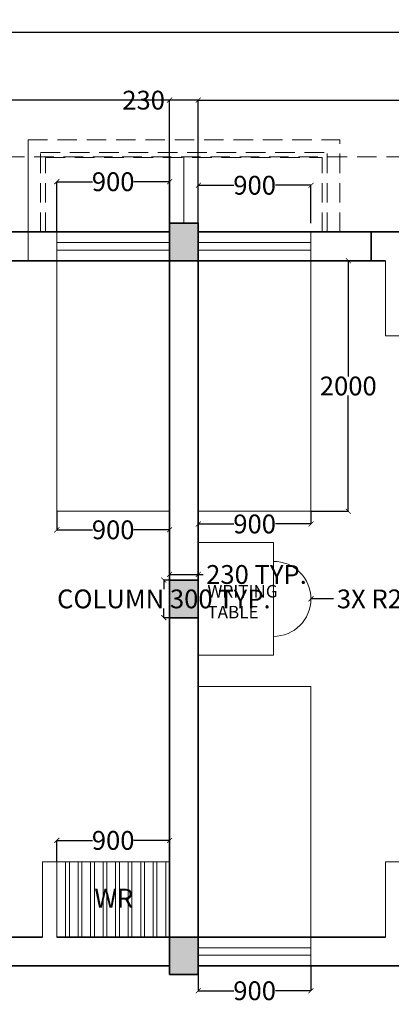
# Model space of a CAD drawing. Units: millimetres. Extents: x 32888 to 53184, y 27889 to 39696.
# Tile 3 of 6: x 38202 to 41170, y 31834 to 39696. Entities that reach past the tile are written whole.
import ezdxf

# ---------------------------------------------------------------- set-up
doc = ezdxf.new("R2010")
doc.units = ezdxf.units.MM
doc.header["$LTSCALE"] = 50
doc.header["$MEASUREMENT"] = 0
doc.linetypes.add('HIDDEN2', pattern=[0.1875, 0.125, -0.0625])
for name, color, linetype, lineweight in [('A-ANNO-DIMS', 2, 'Continuous', 18), ('A-ANNO-TEXT', 7, 'Continuous', 18), ('A-COLS', 1, 'Continuous', 35), ('A-COLS-PATT', 18, 'Continuous', 18), ('A-FURN', 8, 'Continuous', 18), ('A-FURN-CASE', 8, 'Continuous', 18), ('A-GLAZ', 4, 'Continuous', 18), ('A-ROOF', 8, 'Continuous', 18), ('A-ROOF-OVHD', 8, 'HIDDEN2', 18), ('A-WALL', 7, 'Continuous', 35)]:
    doc.layers.add(name, color=color, linetype=linetype, lineweight=lineweight)
doc.styles.get("Standard").update_dxf_attribs({"font": 'arial.ttf'})
doc.dimstyles.get("Standard").update_dxf_attribs({"dimtxt": 150, "dimasz": 40, "dimexe": 0.18, "dimexo": 0.0625, "dimgap": 0.09, "dimtad": 0, "dimtih": 1, "dimtoh": 1, "dimdec": 0, "dimzin": 0, "dimdsep": 46, "dimtxsty": 'Standard', "dimblk": 'ARCHTICK', "dimcen": 0, "dimadec": 0, "dimazin": 0, "dimtfac": 1, "dimtdec": 0, "dimtofl": 0, "dimtmove": 0, "dimatfit": 3, "dimldrblk": 'ARCHTICK', "dimfxl": 1, "dimtolj": 1, "dimtzin": 0, "dimarcsym": 1})

# ---------------------------------------------------------------- blocks, each defined once
blk = doc.blocks.new('_ArchTick')
at = {"color": 0, "linetype": 'ByBlock', "const_width": 0.15}
blk.add_lwpolyline([(-0.5, -0.5), (0.5, 0.5)], dxfattribs=at)
blk = doc.blocks.new('*D14')
at = {"layer": 'A-ANNO-DIMS', "color": 0, "lineweight": -2, "ltscale": 50, "transparency": 16777216}
for p, q in [((38498.9, 32971.1), (38498.9, 33143.1)), ((38498.9, 33142.9), (38783.4, 33142.9)), ((39398.9, 33142.9), (39114.5, 33142.9)), ((39398.9, 32971.1), (39398.9, 33143.1))]:
    blk.add_line(p, q, dxfattribs=at)
at = {"layer": 'Defpoints', "color": 0, "ltscale": 50, "transparency": 16777216}
for p in [(39398.9, 33142.9), (38498.9, 32971), (39398.9, 32971)]:
    blk.add_point(p, dxfattribs=at)
at = {"layer": 'A-ANNO-DIMS', "color": 0, "lineweight": -2, "ltscale": 50, "transparency": 16777216, "xscale": 40, "yscale": 40, "zscale": 40, "rotation": 180}
blk.add_blockref('_ArchTick', (38498.9, 33142.9), dxfattribs=at)
at = {"layer": 'A-ANNO-DIMS', "color": 0, "lineweight": -2, "ltscale": 50, "transparency": 16777216, "xscale": 40, "yscale": 40, "zscale": 40}
blk.add_blockref('_ArchTick', (39398.9, 33142.9), dxfattribs=at)
at = {"layer": 'A-ANNO-DIMS', "color": 0, "ltscale": 50, "transparency": 16777216, "insert": (38948.9, 33142.9), "char_height": 150, "attachment_point": 5}
blk.add_mtext('\\A1;900', dxfattribs=at)
blk = doc.blocks.new('*D18')
at = {"layer": 'A-ANNO-DIMS', "color": 0, "lineweight": -2, "ltscale": 50, "transparency": 16777216}
for p, q in [((39628.9, 32140.9), (39628.9, 31942.1)), ((40528.9, 32140.9), (40528.9, 31942.1)), ((39628.9, 31942.3), (39913.4, 31942.3)), ((40528.9, 31942.3), (40244.5, 31942.3))]:
    blk.add_line(p, q, dxfattribs=at)
at = {"layer": 'Defpoints', "color": 0, "ltscale": 50, "transparency": 16777216}
for p in [(39628.9, 32141), (40528.9, 32141), (40528.9, 31942.3)]:
    blk.add_point(p, dxfattribs=at)
at = {"layer": 'A-ANNO-DIMS', "color": 0, "lineweight": -2, "ltscale": 50, "transparency": 16777216, "xscale": 40, "yscale": 40, "zscale": 40, "rotation": 180}
blk.add_blockref('_ArchTick', (39628.9, 31942.3), dxfattribs=at)
at = {"layer": 'A-ANNO-DIMS', "color": 0, "lineweight": -2, "ltscale": 50, "transparency": 16777216, "xscale": 40, "yscale": 40, "zscale": 40}
blk.add_blockref('_ArchTick', (40528.9, 31942.3), dxfattribs=at)
at = {"layer": 'A-ANNO-DIMS', "color": 0, "ltscale": 50, "transparency": 16777216, "insert": (40078.9, 31942.3), "char_height": 150, "attachment_point": 5}
blk.add_mtext('\\A1;900', dxfattribs=at)
blk = doc.blocks.new('*D36')
at = {"layer": 'A-ANNO-DIMS', "color": 0, "lineweight": -2, "ltscale": 50, "transparency": 16777216}
for p, q in [((40529, 37771), (40826.9, 37771)), ((40826.7, 37771), (40826.7, 36847.7)), ((40826.7, 35771), (40826.7, 36694.3)), ((40529, 35771), (40826.9, 35771))]:
    blk.add_line(p, q, dxfattribs=at)
at = {"layer": 'Defpoints', "color": 0, "ltscale": 50, "transparency": 16777216}
for p in [(40528.9, 37771), (40826.7, 37771), (40528.9, 35771)]:
    blk.add_point(p, dxfattribs=at)
at = {"layer": 'A-ANNO-DIMS', "color": 0, "lineweight": -2, "ltscale": 50, "transparency": 16777216, "xscale": 40, "yscale": 40, "zscale": 40}
for p, rotation in [((40826.7, 37771), 90), ((40826.7, 35771), 270)]:
    blk.add_blockref('_ArchTick', p, dxfattribs=dict(at, rotation=rotation))
at = {"layer": 'A-ANNO-DIMS', "color": 0, "ltscale": 50, "transparency": 16777216, "insert": (40826.7, 36771), "char_height": 150, "attachment_point": 5}
blk.add_mtext('\\A1;2000', dxfattribs=at)
blk = doc.blocks.new('*D37')
at = {"layer": 'A-ANNO-DIMS', "color": 0, "lineweight": -2, "ltscale": 50, "transparency": 16777216}
for p, q in [((39628.9, 35770.9), (39628.9, 35669.2)), ((40528.9, 35770.9), (40528.9, 35669.2)), ((39628.9, 35669.3), (39913.4, 35669.3)), ((40528.9, 35669.3), (40244.5, 35669.3))]:
    blk.add_line(p, q, dxfattribs=at)
at = {"layer": 'Defpoints', "color": 0, "ltscale": 50, "transparency": 16777216}
for p in [(39628.9, 35771), (40528.9, 35771), (39628.9, 35669.3)]:
    blk.add_point(p, dxfattribs=at)
at = {"layer": 'A-ANNO-DIMS', "color": 0, "lineweight": -2, "ltscale": 50, "transparency": 16777216, "xscale": 40, "yscale": 40, "zscale": 40, "rotation": 180}
blk.add_blockref('_ArchTick', (39628.9, 35669.3), dxfattribs=at)
at = {"layer": 'A-ANNO-DIMS', "color": 0, "lineweight": -2, "ltscale": 50, "transparency": 16777216, "xscale": 40, "yscale": 40, "zscale": 40}
blk.add_blockref('_ArchTick', (40528.9, 35669.3), dxfattribs=at)
at = {"layer": 'A-ANNO-DIMS', "color": 0, "ltscale": 50, "transparency": 16777216, "insert": (40078.9, 35669.3), "char_height": 150, "attachment_point": 5}
blk.add_mtext('\\A1;900', dxfattribs=at)
blk = doc.blocks.new('*D38')
at = {"layer": 'A-ANNO-DIMS', "color": 0, "lineweight": -2, "ltscale": 50, "transparency": 16777216}
for p, q in [((38498.9, 35770.9), (38498.9, 35622.5)), ((39398.9, 35770.9), (39398.9, 35622.5)), ((38498.9, 35622.6), (38783.4, 35622.6)), ((39398.9, 35622.6), (39114.5, 35622.6))]:
    blk.add_line(p, q, dxfattribs=at)
at = {"layer": 'Defpoints', "color": 0, "ltscale": 50, "transparency": 16777216}
for p in [(38498.9, 35771), (39398.9, 35771), (38498.9, 35622.6)]:
    blk.add_point(p, dxfattribs=at)
at = {"layer": 'A-ANNO-DIMS', "color": 0, "lineweight": -2, "ltscale": 50, "transparency": 16777216, "xscale": 40, "yscale": 40, "zscale": 40, "rotation": 180.0000000000004}
blk.add_blockref('_ArchTick', (38498.9, 35622.6), dxfattribs=at)
at = {"layer": 'A-ANNO-DIMS', "color": 0, "lineweight": -2, "ltscale": 50, "transparency": 16777216, "xscale": 40, "yscale": 40, "zscale": 40}
blk.add_blockref('_ArchTick', (39398.9, 35622.6), dxfattribs=at)
at = {"layer": 'A-ANNO-DIMS', "color": 0, "ltscale": 50, "transparency": 16777216, "insert": (38948.9, 35622.6), "char_height": 150, "attachment_point": 5}
blk.add_mtext('\\A1;900', dxfattribs=at)
blk = doc.blocks.new('*D45')
at = {"layer": 'A-ANNO-DIMS', "color": 0, "lineweight": -2, "ltscale": 50, "transparency": 16777216}
for p, q in [((39628.9, 38071.1), (39628.9, 38373.9)), ((39628.9, 38373.7), (39913.4, 38373.7)), ((40528.9, 38373.7), (40244.5, 38373.7)), ((40528.9, 38071.1), (40528.9, 38373.9))]:
    blk.add_line(p, q, dxfattribs=at)
at = {"layer": 'Defpoints', "color": 0, "ltscale": 50, "transparency": 16777216}
for p in [(40528.9, 38373.7), (39628.9, 38071), (40528.9, 38071)]:
    blk.add_point(p, dxfattribs=at)
at = {"layer": 'A-ANNO-DIMS', "color": 0, "lineweight": -2, "ltscale": 50, "transparency": 16777216, "xscale": 40, "yscale": 40, "zscale": 40, "rotation": 180}
blk.add_blockref('_ArchTick', (39628.9, 38373.7), dxfattribs=at)
at = {"layer": 'A-ANNO-DIMS', "color": 0, "lineweight": -2, "ltscale": 50, "transparency": 16777216, "xscale": 40, "yscale": 40, "zscale": 40}
blk.add_blockref('_ArchTick', (40528.9, 38373.7), dxfattribs=at)
at = {"layer": 'A-ANNO-DIMS', "color": 0, "ltscale": 50, "transparency": 16777216, "insert": (40078.9, 38373.7), "char_height": 150, "attachment_point": 5}
blk.add_mtext('\\A1;900', dxfattribs=at)
blk = doc.blocks.new('*D46')
at = {"layer": 'A-ANNO-DIMS', "color": 0, "lineweight": -2, "ltscale": 50, "transparency": 16777216}
for p, q in [((38498.9, 38001.1), (38498.9, 38402)), ((38498.9, 38401.9), (38783.4, 38401.9)), ((39398.9, 38401.9), (39114.5, 38401.9)), ((39398.9, 38001.1), (39398.9, 38402))]:
    blk.add_line(p, q, dxfattribs=at)
at = {"layer": 'Defpoints', "color": 0, "ltscale": 50, "transparency": 16777216}
for p in [(39398.9, 38401.9), (38498.9, 38001), (39398.9, 38001)]:
    blk.add_point(p, dxfattribs=at)
at = {"layer": 'A-ANNO-DIMS', "color": 0, "lineweight": -2, "ltscale": 50, "transparency": 16777216, "xscale": 40, "yscale": 40, "zscale": 40, "rotation": 180}
blk.add_blockref('_ArchTick', (38498.9, 38401.9), dxfattribs=at)
at = {"layer": 'A-ANNO-DIMS', "color": 0, "lineweight": -2, "ltscale": 50, "transparency": 16777216, "xscale": 40, "yscale": 40, "zscale": 40}
blk.add_blockref('_ArchTick', (39398.9, 38401.9), dxfattribs=at)
at = {"layer": 'A-ANNO-DIMS', "color": 0, "ltscale": 50, "transparency": 16777216, "insert": (38948.9, 38401.9), "char_height": 150, "attachment_point": 5}
blk.add_mtext('\\A1;900', dxfattribs=at)
blk = doc.blocks.new('*D52')
at = {"layer": 'A-ANNO-DIMS', "color": 0, "lineweight": -2, "ltscale": 50, "transparency": 16777216}
for p, q in [((39628.9, 38001.1), (39628.9, 39053.3)), ((39628.9, 39053.1), (41355.2, 39053.1)), ((43528.9, 39053.1), (41802.7, 39053.1)), ((43528.9, 38001.1), (43528.9, 39053.3))]:
    blk.add_line(p, q, dxfattribs=at)
at = {"layer": 'Defpoints', "color": 0, "ltscale": 50, "transparency": 16777216}
for p in [(39628.9, 39053.1), (39628.9, 38001), (43528.9, 38001)]:
    blk.add_point(p, dxfattribs=at)
at = {"layer": 'A-ANNO-DIMS', "color": 0, "lineweight": -2, "ltscale": 50, "transparency": 16777216, "xscale": 40, "yscale": 40, "zscale": 40, "rotation": 180}
blk.add_blockref('_ArchTick', (39628.9, 39053.1), dxfattribs=at)
at = {"layer": 'A-ANNO-DIMS', "color": 0, "lineweight": -2, "ltscale": 50, "transparency": 16777216, "xscale": 40, "yscale": 40, "zscale": 40}
blk.add_blockref('_ArchTick', (43528.9, 39053.1), dxfattribs=at)
at = {"layer": 'A-ANNO-DIMS', "color": 0, "ltscale": 50, "transparency": 16777216, "insert": (41578.9, 39053.1), "char_height": 150, "attachment_point": 5}
blk.add_mtext('\\A1;3900', dxfattribs=at)
blk = doc.blocks.new('*D53')
at = {"layer": 'A-ANNO-DIMS', "color": 0, "lineweight": -2, "ltscale": 50, "transparency": 16777216}
for p, q in [((39398.9, 39053.3), (39358.9, 39053.3)), ((39398.9, 38071.1), (39398.9, 39053.5)), ((39628.9, 39053.3), (39398.9, 39053.3)), ((39628.9, 38071.1), (39628.9, 39053.5))]:
    blk.add_line(p, q, dxfattribs=at)
at = {"layer": 'Defpoints', "color": 0, "ltscale": 50, "transparency": 16777216}
for p in [(39398.9, 39053.3), (39398.9, 38071), (39628.9, 38071)]:
    blk.add_point(p, dxfattribs=at)
at = {"layer": 'A-ANNO-DIMS', "color": 0, "lineweight": -2, "ltscale": 50, "transparency": 16777216, "xscale": 40, "yscale": 40, "zscale": 40}
for p, rotation in [((39398.9, 39053.3), 179.9999999999819), ((39628.9, 39053.3), 359.9999999999819)]:
    blk.add_blockref('_ArchTick', p, dxfattribs=dict(at, rotation=rotation))
at = {"layer": 'A-ANNO-DIMS', "color": 0, "ltscale": 50, "transparency": 16777216, "insert": (39192.1, 39053.3), "char_height": 150, "attachment_point": 5}
blk.add_mtext('\\A1;230', dxfattribs=at)
blk = doc.blocks.new('*D54')
at = {"layer": 'A-ANNO-DIMS', "color": 0, "lineweight": -2, "ltscale": 50, "transparency": 16777216}
for p, q in [((35398.9, 38001.1), (35398.9, 39053.1)), ((35398.9, 39052.9), (37172.1, 39052.9)), ((39398.9, 39052.9), (37625.8, 39052.9)), ((39398.9, 38001.1), (39398.9, 39053.1))]:
    blk.add_line(p, q, dxfattribs=at)
at = {"layer": 'Defpoints', "color": 0, "ltscale": 50, "transparency": 16777216}
for p in [(35398.9, 39052.9), (35398.9, 38001), (39398.9, 38001)]:
    blk.add_point(p, dxfattribs=at)
at = {"layer": 'A-ANNO-DIMS', "color": 0, "lineweight": -2, "ltscale": 50, "transparency": 16777216, "xscale": 40, "yscale": 40, "zscale": 40, "rotation": 180}
blk.add_blockref('_ArchTick', (35398.9, 39052.9), dxfattribs=at)
at = {"layer": 'A-ANNO-DIMS', "color": 0, "lineweight": -2, "ltscale": 50, "transparency": 16777216, "xscale": 40, "yscale": 40, "zscale": 40}
blk.add_blockref('_ArchTick', (39398.9, 39052.9), dxfattribs=at)
at = {"layer": 'A-ANNO-DIMS', "color": 0, "ltscale": 50, "transparency": 16777216, "insert": (37398.9, 39052.9), "char_height": 150, "attachment_point": 5}
blk.add_mtext('\\A1;4000', dxfattribs=at)
blk = doc.blocks.new('*D57')
at = {"layer": 'A-ANNO-DIMS', "color": 0, "lineweight": -2, "ltscale": 50, "transparency": 16777216}
for p, q in [((35168.9, 38001.1), (35168.9, 39597.3)), ((35168.9, 39597.2), (42753.9, 39597.2)), ((50888.9, 39597.2), (43304, 39597.2)), ((50888.9, 38001.1), (50888.9, 39597.3))]:
    blk.add_line(p, q, dxfattribs=at)
at = {"layer": 'Defpoints', "color": 0, "ltscale": 50, "transparency": 16777216}
for p in [(50888.9, 39597.2), (35168.9, 38001), (50888.9, 38001)]:
    blk.add_point(p, dxfattribs=at)
at = {"layer": 'A-ANNO-DIMS', "color": 0, "lineweight": -2, "ltscale": 50, "transparency": 16777216, "xscale": 40, "yscale": 40, "zscale": 40, "rotation": 180}
blk.add_blockref('_ArchTick', (35168.9, 39597.2), dxfattribs=at)
at = {"layer": 'A-ANNO-DIMS', "color": 0, "lineweight": -2, "ltscale": 50, "transparency": 16777216, "xscale": 40, "yscale": 40, "zscale": 40}
blk.add_blockref('_ArchTick', (50888.9, 39597.2), dxfattribs=at)
at = {"layer": 'A-ANNO-DIMS', "color": 0, "ltscale": 50, "transparency": 16777216, "insert": (43028.9, 39597.2), "char_height": 150, "attachment_point": 5}
blk.add_mtext('\\A1;15720', dxfattribs=at)
blk = doc.blocks.new('BED-SINGLE-900')
for p in [(900, 2230), (0, 0)]:
    blk.add_line(p, (900, 0))
blk = doc.blocks.new('DESK-WITH-CHAIR-900')
for p, q in [((0, 299.6), (0, 899.6)), ((900, 899.6), (900, 299.6)), ((900, 299.6), (0, 299.6))]:
    blk.add_line(p, q)
blk.add_arc((450, 299.6), 299.6, 180, 0)
blk = doc.blocks.new('WARDROBE-SLATTED-PANEL-900')
at = {"ltscale": 50}
for p, q in [((-830, 600), (-830, 0)), ((-800, 600), (-800, 0)), ((-730, 600), (-730, 0)), ((-700, 600), (-700, 0)), ((-630, 600), (-630, 0)), ((-600, 600), (-600, 0)), ((-530, 600), (-530, 0)), ((-500, 600), (-500, 0)), ((-430, 600), (-430, 0)), ((-400, 600), (-400, 0)), ((-330, 600), (-330, 0)), ((-300, 600), (-300, 0)), ((-230, 600), (-230, 0)), ((-200, 600), (-200, 0)), ((-130, 600), (-130, 0)), ((-100, 600), (-100, 0)), ((-30, 600), (-30, 0)), ((-30, 0), (0, 0))]:
    blk.add_line(p, q, dxfattribs=at)
blk = doc.blocks.new('WINDOW-900')
for p, q in [((900, 60), (0, 60)), ((900, 0), (0, 0))]:
    blk.add_line(p, q)
blk = doc.blocks.new('COLUMN-IN-WALL-230x300')
for points in [[(0, 300), (230, 300)], [(230, 0), (0, 0)]]:
    blk.add_lwpolyline(points)
blk = doc.blocks.new('*D73')
at = {"layer": 'A-ANNO-DIMS', "color": 0, "lineweight": -2, "ltscale": 50, "transparency": 16777216}
for p, q in [((39398.9, 35221), (39353.8, 35221)), ((39353.9, 35221), (39353.9, 35148.8)), ((39353.9, 34921), (39353.9, 34993.3)), ((39398.9, 34921), (39353.8, 34921))]:
    blk.add_line(p, q, dxfattribs=at)
at = {"layer": 'Defpoints', "color": 0, "ltscale": 50, "transparency": 16777216}
for p in [(39353.9, 35221), (39398.9, 35221), (39398.9, 34921)]:
    blk.add_point(p, dxfattribs=at)
at = {"layer": 'A-ANNO-DIMS', "color": 0, "lineweight": -2, "ltscale": 50, "transparency": 16777216, "xscale": 40, "yscale": 40, "zscale": 40}
for p, rotation in [((39353.9, 35221), 90), ((39353.9, 34921), 270)]:
    blk.add_blockref('_ArchTick', p, dxfattribs=dict(at, rotation=rotation))
at = {"layer": 'A-ANNO-DIMS', "color": 0, "ltscale": 50, "transparency": 16777216, "insert": (39353.9, 35071), "char_height": 150, "attachment_point": 5}
blk.add_mtext('\\A1;COLUMN 300 TYP.', dxfattribs=at)
blk = doc.blocks.new('*D74')
at = {"layer": 'A-ANNO-DIMS', "color": 0, "lineweight": -2, "ltscale": 50, "transparency": 16777216}
for p, q in [((39398.9, 35221.1), (39398.9, 35266.2)), ((39398.9, 35266), (39628.9, 35266)), ((39628.9, 35221.1), (39628.9, 35266.2)), ((39628.9, 35266), (39668.9, 35266))]:
    blk.add_line(p, q, dxfattribs=at)
at = {"layer": 'Defpoints', "color": 0, "ltscale": 50, "transparency": 16777216}
for p in [(39398.9, 35221), (39628.9, 35266), (39628.9, 35221)]:
    blk.add_point(p, dxfattribs=at)
at = {"layer": 'A-ANNO-DIMS', "color": 0, "lineweight": -2, "ltscale": 50, "transparency": 16777216, "xscale": 40, "yscale": 40, "zscale": 40, "rotation": 180}
blk.add_blockref('_ArchTick', (39398.9, 35266), dxfattribs=at)
at = {"layer": 'A-ANNO-DIMS', "color": 0, "lineweight": -2, "ltscale": 50, "transparency": 16777216, "xscale": 40, "yscale": 40, "zscale": 40}
blk.add_blockref('_ArchTick', (39628.9, 35266), dxfattribs=at)
at = {"layer": 'A-ANNO-DIMS', "color": 0, "ltscale": 50, "transparency": 16777216, "insert": (40093.7, 35266), "char_height": 150, "attachment_point": 5}
blk.add_mtext('\\A1;230 TYP.', dxfattribs=at)
blk = doc.blocks.new('*D81')
at = {"layer": 'A-ANNO-DIMS', "color": 0, "lineweight": -2, "ltscale": 50, "transparency": 16777216}
blk.add_line((40708.3, 35071), (40528.5, 35071), dxfattribs=at)
at = {"layer": 'Defpoints', "color": 0, "ltscale": 50, "transparency": 16777216}
for p in [(40228.9, 35071), (40528.5, 35071)]:
    blk.add_point(p, dxfattribs=at)
at = {"layer": 'A-ANNO-DIMS', "color": 0, "lineweight": -2, "ltscale": 50, "transparency": 16777216, "xscale": 40, "yscale": 40, "zscale": 40, "rotation": 180.0000030600586}
blk.add_blockref('_ArchTick', (40528.5, 35071), dxfattribs=at)
at = {"layer": 'A-ANNO-DIMS', "color": 0, "ltscale": 50, "transparency": 16777216, "insert": (41194.3, 35071), "char_height": 150, "attachment_point": 5}
blk.add_mtext('\\A1;3X R299.6', dxfattribs=at)

msp = doc.modelspace()

# ---------------------------------------------------------------- hatches: boundary and pattern name
at = {"layer": 'A-COLS-PATT', "ltscale": 50}
h = msp.add_hatch(color=256, dxfattribs=at)
h.dxf.hatch_style = 1
h.paths.add_polyline_path([(35398.95, 38071.01), (35168.95, 38071.01), (35168.95, 37771.01), (35398.95, 37771.01)])
h.paths.add_polyline_path([(39628.95, 38071.01), (39398.95, 38071.01), (39398.95, 37771.01), (39628.95, 37771.01)])
h.paths.add_polyline_path([(43903.95, 38071.01), (43673.95, 38071.01), (43673.95, 37771.01), (43903.95, 37771.01)])
h.paths.add_polyline_path([(47658.95, 38071.01), (47428.95, 38071.01), (47428.95, 37771.01), (47658.95, 37771.01)])
h.paths.add_polyline_path([(50888.95, 38071.01), (50658.95, 38071.01), (50658.95, 37771.01), (50888.95, 37771.01)])
h.paths.add_polyline_path([(50888.95, 35221.01), (50658.95, 35221.01), (50658.95, 34921.01), (50888.95, 34921.01)])
h.paths.add_polyline_path([(47658.95, 35221.01), (47428.95, 35221.01), (47428.95, 34921.01), (47658.95, 34921.01)])
h.paths.add_polyline_path([(39628.95, 35071.01), (39628.95, 35221.01), (39398.95, 35221.01), (39398.95, 34921.01), (39628.95, 34921.01)])
h.paths.add_polyline_path([(35398.95, 35221.01), (35168.95, 35221.01), (35168.95, 34921.01), (35398.95, 34921.01)])
h.paths.add_polyline_path([(35398.95, 32371.01), (35168.95, 32371.01), (35168.95, 32071.01), (35398.95, 32071.01)])
h.paths.add_polyline_path([(35418.95, 30571.01), (35168.95, 30571.01), (35168.95, 30271.01), (35418.95, 30271.01)])
h.paths.add_polyline_path([(39642.61, 30571.01), (39392.61, 30571.01), (39392.61, 30271.01), (39642.61, 30271.01)])
h.paths.add_polyline_path([(39628.95, 32371.01), (39398.95, 32371.01), (39398.95, 32071.01), (39628.95, 32071.01)])
h.paths.add_polyline_path([(43903.95, 32371.01), (43673.95, 32371.01), (43673.95, 32071.01), (43903.95, 32071.01)])
h.paths.add_polyline_path([(43903.95, 30571.01), (43653.95, 30571.01), (43653.95, 30271.01), (43903.95, 30271.01)])
h.paths.add_polyline_path([(47658.95, 32441.01), (47428.95, 32441.01), (47428.95, 32141.01), (47658.95, 32141.01)])
h.paths.add_polyline_path([(50888.95, 32414.45), (50658.95, 32414.45), (50658.95, 32114.45), (50888.95, 32114.45)])
h.paths.add_polyline_path([(50888.95, 30571.01), (50638.95, 30571.01), (50638.95, 30271.01), (50888.95, 30271.01)])
h.paths.add_polyline_path([(47678.95, 30571.01), (47428.95, 30571.01), (47428.95, 30341.01), (47678.95, 30341.01)])
h.paths.add_polyline_path([(47678.95, 30341.01), (47428.95, 30341.01), (47428.95, 30271.01), (47678.95, 30271.01)])

# ---------------------------------------------------------------- linework, layer by layer
at = {"layer": 'A-COLS'}
for points in [[(39398.95, 38071.01), (39628.95, 38071.01)], [(39628.95, 32071.01), (39398.95, 32071.01)]]:
    msp.add_lwpolyline(points, dxfattribs=at)
at = {"layer": 'A-FURN-CASE'}
for p, q in [((41123.95, 37171.01), (41123.95, 37771.01)), ((44383.95, 37171.01), (41123.95, 37171.01)), ((38383.95, 32371.01), (38383.95, 32971.01)), ((38498.95, 32371.01), (38498.95, 32971.01)), ((41123.95, 32971.01), (41123.95, 32371.01)), ((42253.95, 32971.01), (41123.95, 32971.01))]:
    msp.add_line(p, q, dxfattribs=at)
at = {"layer": 'A-FURN-CASE', "ltscale": 50}
msp.add_line((38383.95, 32971.01), (39398.95, 32971.01), dxfattribs=at)
at = {"layer": 'A-ROOF'}
for p, q in [((38268.95, 37771.01), (38268.95, 38736.01)), ((39513.95, 38071.01), (39513.95, 38596.01))]:
    msp.add_line(p, q, dxfattribs=at)
at = {"layer": 'A-ROOF-OVHD', "ltscale": 25}
for p, q in [((38268.95, 38736.01), (40758.95, 38736.01)), ((40758.95, 38001.01), (40758.95, 38736.01)), ((34568.95, 38601.01), (51488.95, 38601.01)), ((38368.95, 38636.01), (40658.95, 38636.01)), ((38368.95, 38001.01), (38368.95, 38636.01)), ((40658.95, 38001.01), (40658.95, 38636.01)), ((38408.95, 38596.01), (40618.95, 38596.01)), ((38408.95, 38001.01), (38408.95, 38596.01)), ((40618.95, 38001.01), (40618.95, 38596.01))]:
    msp.add_line(p, q, dxfattribs=at)
at = {"layer": 'A-WALL'}
for p, q in [((39398.95, 38596.01), (39398.95, 32071.01)), ((35398.95, 38001.01), (39398.95, 38001.01)), ((39628.95, 38001.01), (43673.95, 38001.01)), ((41008.95, 37771.01), (41008.95, 38001.01)), ((37671.2, 32371.01), (38383.95, 32371.01)), ((38498.95, 32371.01), (41123.95, 32371.01)), ((37671.2, 32141.01), (39398.95, 32141.01)), ((39628.95, 32141.01), (43673.95, 32141.01))]:
    msp.add_line(p, q, dxfattribs=at)
for points in [[(39628.95, 32071.01), (39628.95, 38071.01)], [(35168.95, 37771.01), (41123.95, 37771.01)]]:
    msp.add_lwpolyline(points, dxfattribs=at)

# ---------------------------------------------------------------- block references
at = {"layer": 'A-COLS'}
msp.add_blockref('COLUMN-IN-WALL-230x300', (39398.95, 34921.01), dxfattribs=at)
at = {"layer": 'A-FURN', "extrusion": (0, 0, -1), "zscale": -1}
msp.add_blockref('BED-SINGLE-900', (-39398.95, 35771.01), dxfattribs=at)
at = {"layer": 'A-FURN'}
msp.add_blockref('BED-SINGLE-900', (39628.95, 35771.01), dxfattribs=at)
at = {"layer": 'A-FURN', "rotation": 89.99999999999866}
msp.add_blockref('DESK-WITH-CHAIR-900', (40528.53, 34621.01), dxfattribs=at)
at = {"layer": 'A-FURN', "extrusion": (0, 0, -1), "zscale": -1, "rotation": 180}
msp.add_blockref('BED-SINGLE-900', (-39628.95, 34371.01), dxfattribs=at)
at = {"layer": 'A-FURN-CASE'}
msp.add_blockref('WARDROBE-SLATTED-PANEL-900', (39398.95, 32371.01), dxfattribs=at)
at = {"layer": 'A-GLAZ', "rotation": 180}
for p in [(39398.95, 37916.01), (40528.95, 37916.01)]:
    msp.add_blockref('WINDOW-900', p, dxfattribs=at)
at = {"layer": 'A-GLAZ'}
msp.add_blockref('WINDOW-900', (39628.95, 32226.01), dxfattribs=at)

# ---------------------------------------------------------------- texts
at = {"layer": 'A-ANNO-TEXT', "ltscale": 50, "attachment_point": 1}
for s, width, insert, char_height in [('WRITING\\PTABLE', 901.3249, (39701.48, 35182.05), 100), ('WR', 742.516, (38798.95, 32756.82), 150)]:
    msp.add_mtext_dynamic_manual_height_columns(s, width=width, gutter_width=1, heights=[0], dxfattribs=dict(at, insert=insert, char_height=char_height))

# ---------------------------------------------------------------- dimensions: what is measured, and where the dimension line sits
at = {"layer": 'A-ANNO-DIMS', "ltscale": 50}
for p1, p2, distance, picture, middle in [((35168.95, 38001.01), (50888.95, 38001.01), 1596.15, '*D57', (43028.95, 39597.16)), ((39398.95, 38001.01), (35398.95, 38001.01), -1051.9, '*D54', (37398.95, 39052.91)), ((39628.95, 38071.01), (39398.95, 38071.01), -982.26, '*D53', (39192.13, 39053.27)), ((43528.95, 38001.01), (39628.95, 38001.01), -1052.08, '*D52', (41578.95, 39053.09)), ((38498.95, 38001.01), (39398.95, 38001.01), 400.85, '*D46', (38948.95, 38401.86)), ((39628.95, 38071.01), (40528.95, 38071.01), 302.68, '*D45', (40078.95, 38373.69)), ((40528.95, 35771.01), (40528.95, 37771.01), -297.77, '*D36', (40826.72, 36771.01)), ((39398.95, 35771.01), (38498.95, 35771.01), 148.37, '*D38', (38948.95, 35622.64)), ((40528.95, 35771.01), (39628.95, 35771.01), 101.67, '*D37', (40078.95, 35669.34)), ((38498.95, 32971.01), (39398.95, 32971.01), 171.94, '*D14', (38948.95, 33142.94)), ((39628.95, 32141.01), (40528.95, 32141.01), -198.73, '*D18', (40078.95, 31942.28))]:
    dim = msp.add_aligned_dim(p1=p1, p2=p2, distance=distance, dimstyle='Standard', override={"dimclrd": 0, "dimclre": 0, "dimclrt": 0}, dxfattribs=at)
    dim.commit()
    dim.dimension.update_dxf_attribs({"geometry": picture, "text_midpoint": middle})
dim = msp.add_linear_dim(base=(39628.95, 35266.01), p1=(39398.95, 35221.01), p2=(39628.95, 35221.01), text='<> TYP.', dimstyle='Standard', override={"dimdec": 0, "dimlfac": 1, "dimrnd": 0, "dimzin": 0, "dimdsep": 46, "dimlunit": 2}, dxfattribs=at)
dim.commit()
dim.dimension.update_dxf_attribs({"geometry": '*D74', "text_midpoint": (40093.66, 35266.01)})
dim = msp.add_linear_dim(base=(39353.95, 35221.01), p1=(39398.95, 34921.01), p2=(39398.95, 35221.01), angle=90, text='COLUMN <> TYP.', dimstyle='Standard', override={"dimdec": 0, "dimlfac": 1, "dimrnd": 0, "dimzin": 0, "dimdsep": 46, "dimlunit": 2}, dxfattribs=at)
dim.commit()
dim.dimension.update_dxf_attribs({"geometry": '*D73', "text_midpoint": (39353.95, 35071.01)})
dim = msp.add_radius_dim(center=(40228.95, 35071.01), mpoint=(40528.53, 35071.01), text='3X <>', dimstyle='Standard', override={"dimdec": 1, "dimlfac": 1, "dimrnd": 0, "dimzin": 0, "dimdsep": 46, "dimlunit": 2}, dxfattribs=at)
dim.commit()
dim.dimension.update_dxf_attribs({"geometry": '*D81', "text_midpoint": (40708.28, 35071.01), "dimtype": 164})

doc.saveas('drawing.dxf')
